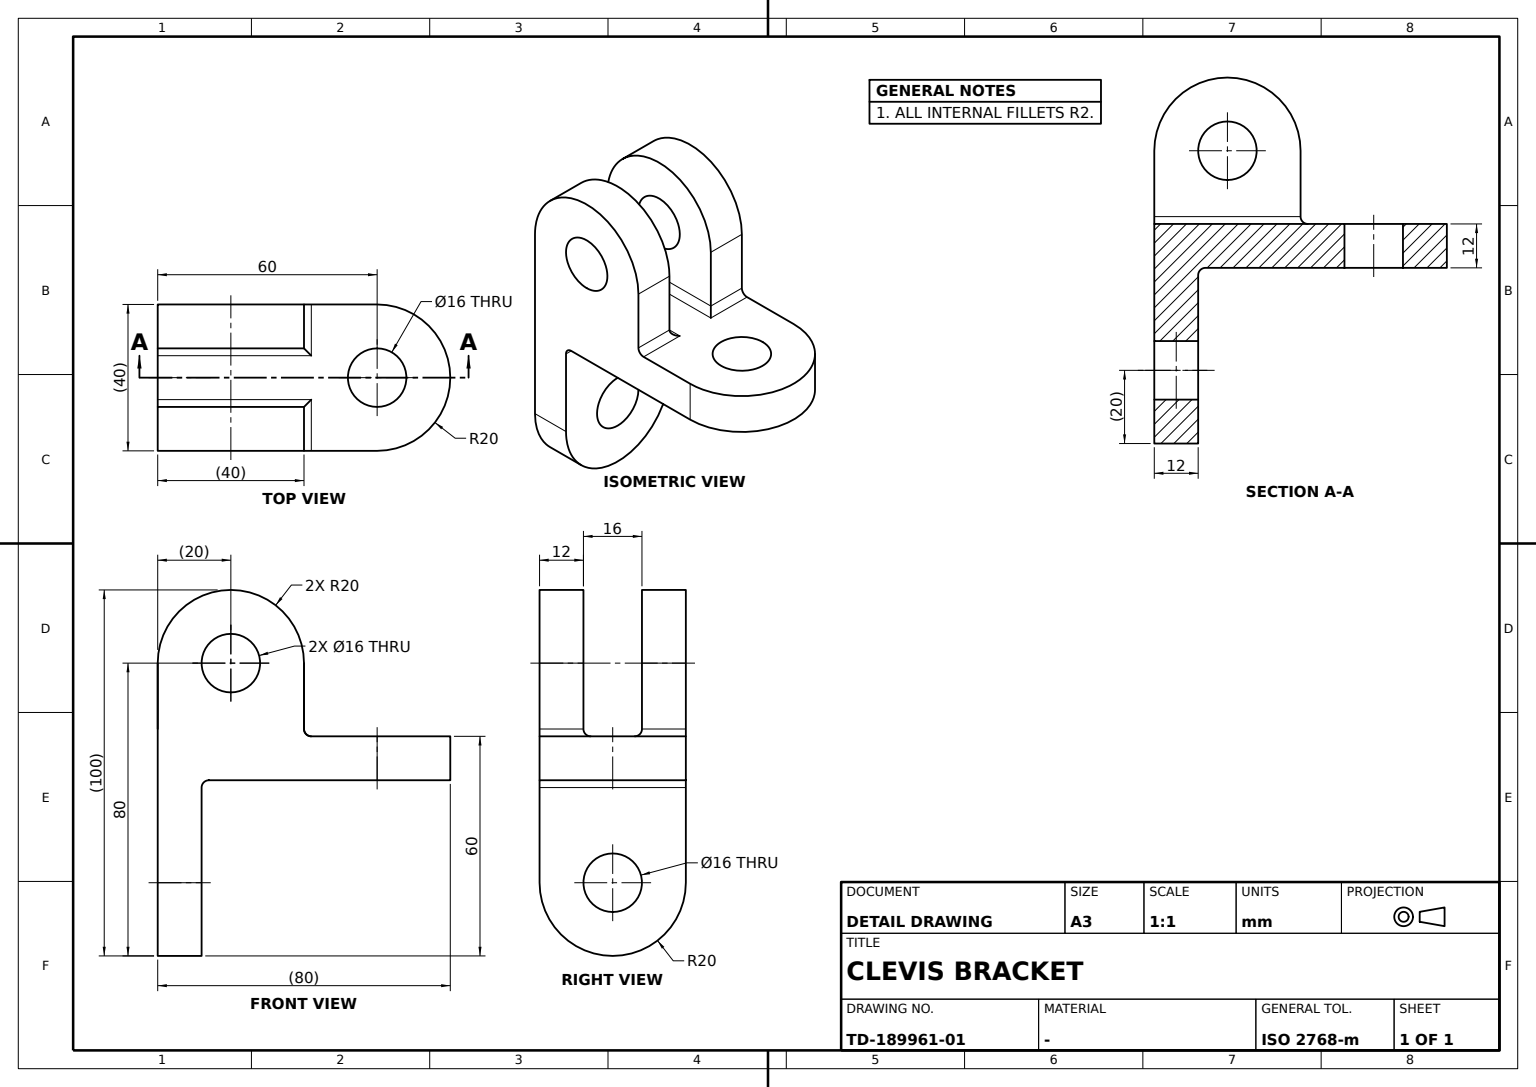
CATIA V5 part; units mm, degrees
sketch "Sketch1" plane through (0, 0, 0) normal (1, 0, 0) x (0, 1, 0)
  line L0 (0, 0) -> (0, 50)
  arc A0 (0, 50) -> (40, 50) centre (20, 50) cw
  point P0 (20, 50)
  line L1 (40, 50) -> (40, 30)
  line L2 (40, 30) -> (60, 30)
  line L3 (60, 30) -> (60, 18)
  line L4 (60, 18) -> (12, 18)
  line L5 (12, 18) -> (12, -10)
  line L6 (12, -10) -> (0, -10)
  point P1 (0, -10)
  line L7 (0, -10) -> (0, 0)
  dimension "radius A0" = 20
  dimension "length L2" = 20
  dimension "distance L2 L4" = 12
  dimension "distance P0 L6" = 60
  dimension "distance L7 L5" = 12
  dimension "distance P0 L2" = 20
  constraint vertical L0 y-axis
  constraint vertical L3 y-axis
  constraint vertical L5 y-axis
  constraint tangency A0 L0
  constraint tangency L1 A0
  constraint tangency L7 A0
  constraint horizontal L2 x-axis
  constraint horizontal L4 x-axis
  constraint horizontal L6 x-axis
  constraint coincidence P1 y-axis
extrude "Pad1" add sketch "Sketch1" along normal mid plane 40
sketch "Sketch2" plane through (0, 0, 30) normal (0, 0, 1) x (1, 0, 0)
  line L0 (-20, 60) -> (20, 60)
  arc A0 (20, 60) -> (-20, 60) centre (0, 60) ccw
  point P0 (0, 60)
  constraint coincidence P0 y-axis
  constraint coincidence P0 L0
extrude "Pad2" add sketch "Sketch2" against normal blind 12
sketch "Sketch3" plane through (0, 12, 0) normal (0, 1, 0) x (-1, 0, 0)
  line L0 (20, -10) -> (-20, -10)
  arc A0 (-20, -10) -> (20, -10) centre (0, -10) ccw
  point P0 (0, -10)
  constraint coincidence P0 L0
extrude "Pad3" add sketch "Sketch3" against normal blind 12
sketch "Sketch4" plane through (20, 18.3156, 50) normal (1, 0, 0) x (0, 1, 0)
  point P0 (1.6844, 0)
  arc A0 (21.6844, 0) -> (-18.3156, 0) centre (1.6844, 0) ccw construction
  constraint concentricity P0 A0
hole "Hole1" at (20, 20, 50) direction (-1, 0, 0) diameter 16 depth 40
sketch "Sketch5" plane through (-1.2987, 56.7211, 30) normal (0, 0, 1) x (1, 0, 0)
  point P0 (1.2987, 3.2789)
  arc A0 (21.2987, 3.2789) -> (-18.7013, 3.2789) centre (1.2987, 3.2789) ccw construction
  constraint concentricity P0 A0
hole "Hole2" at (0, 60, 30) direction (0, 0, -1) diameter 16 depth 40
sketch "Sketch6" plane through (-2.7758, 12, -14.3726) normal (0, 1, 0) x (1, 0, 0)
  point P0 (2.7758, -4.3726)
  arc A0 (22.7758, -4.3726) -> (-17.2242, -4.3726) centre (2.7758, -4.3726) ccw construction
  constraint concentricity P0 A0
hole "Hole3" at (0, 12, -10) direction (0, -1, 0) diameter 16 depth 12
sketch "Sketch7" plane through (0, 40, 0) normal (0, 1, 0) x (-1, 0, 0)
  line L0 (-8, 90) -> (8, 90)
  line L1 (8, 90) -> (8, 30)
  line L2 (8, 30) -> (-8, 30)
  line L3 (-8, 30) -> (-8, 90)
  line L4 (-20, 30) -> (20, 30) construction
  dimension "distance L3 L1" = 16
  constraint horizontal L0 x-axis
  constraint horizontal L2 x-axis
  constraint vertical L1 y-axis
  constraint vertical L3 y-axis
  constraint coincidence L2 L4
  constraint symmetry L3 L1 y-axis
extrude "Pocket1" cut sketch "Sketch7" against normal blind 40
fillet "Fillet1" radius 2 2 edges at (14, 40, 30) (-14, 40, 30)
fillet "Fillet2" radius 2 2 edges at (-8, 20, 30) (8, 20, 30)
fillet "Fillet3" radius 2 1 edges at (0, 12, 18)
